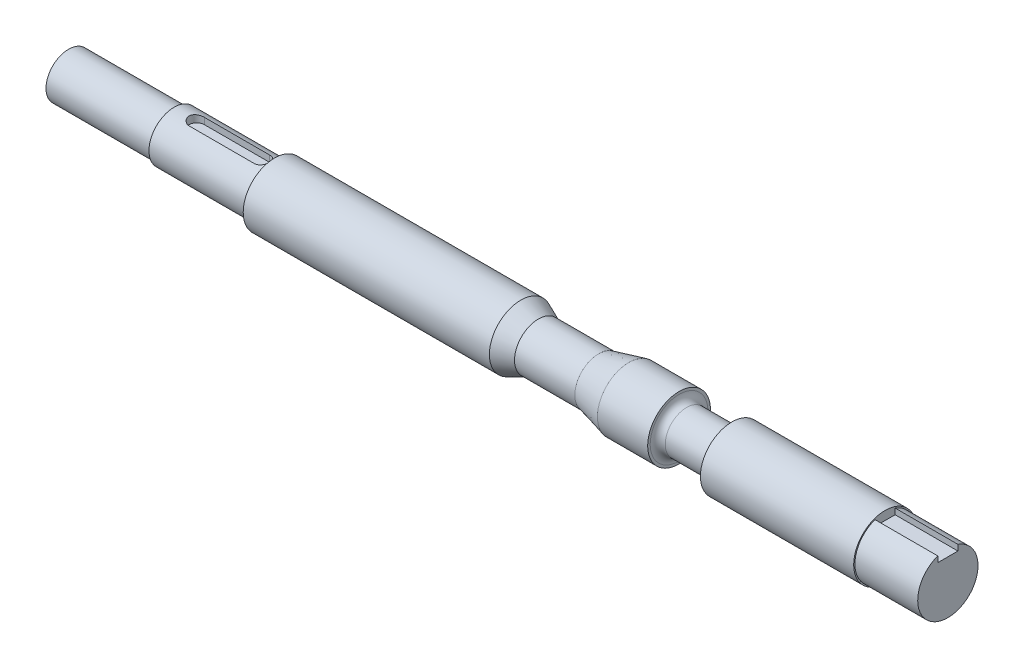
SolidWorks part; units mm, degrees
material "Plain Carbon Steel"
ref_plane "Front Plane" through (0, 0, 0) normal (0, 0, 1) x (1, 0, 0)
ref_plane "Top Plane" through (0, 0, 0) normal (0, 1, 0) x (1, 0, 0)
ref_plane "Right Plane" through (0, 0, 0) normal (1, 0, 0) x (0, 0, -1)
sketch "Shaft Profile Sketch" plane through (0, 0, 0) normal (0, 0, 1) x (1, 0, 0)
  line L0 (0, 0) -> (350, 0)
  line L1 (350, 0) -> (350, 12)
  line L2 (350, 12) -> (325, 12)
  line L3 (325, 12) -> (325, 12.5)
  line L4 (325, 12.5) -> (264, 12.5)
  line L5 (243, 12.5) -> (243, 8.5)
  line L6 (243, 8.5) -> (264, 8.5)
  line L7 (264, 8.5) -> (264, 12.5)
  line L8 (243, 12.5) -> (223, 12.5)
  line L9 (223, 12.5) -> (211, 9.5)
  line L10 (211, 9.5) -> (187, 9.5)
  line L11 (187, 9.5) -> (180, 12.5)
  line L12 (180, 12.5) -> (82, 12.5)
  line L13 (82, 12.5) -> (82, 10)
  line L14 (82, 10) -> (42, 10)
  line L15 (42, 10) -> (42, 9)
  line L16 (42, 9) -> (0, 9)
  line L17 (0, 9) -> (0, 0)
  dimension "D1" = 350
  dimension "D2" = 12
  dimension "D3" = 12.5
  dimension "D4" = 8.5
  dimension "D5" = 9
  dimension "D6" = 10
  dimension "D7" = 9.5
  dimension "D8" = 86
  dimension "D9" = 25
  dimension "D10" = 107
  dimension "D11" = 20
  dimension "D12" = 12
  dimension "D13" = 31
  dimension "D14" = 7
  dimension "D15" = 98
  dimension "D16" = 40
revolve "Shaft Body Revolve" add sketch "Shaft Profile Sketch" angle 360 about L0
fillet "Shoulder Fillet R2" radius 2 1 edges at (264, 0, 8.5)
fillet "Shoulder Fillet R3" radius 3 1 edges at (243, 0, 8.5)
sketch "Keyway A Sketch" plane through (350, 0, 0) normal (1, 0, 0) x (0, 0, -1)
  line L1 (-4, 9) -> (4, 9)
  line L2 (-4, 9) -> (-4, 15)
  line L3 (-4, 15) -> (4, 15)
  line L4 (4, 9) -> (4, 15)
  line L5 (-4, 9) -> (4, 15) construction
  line L6 (-4, 15) -> (4, 9) construction
  circle A0 centre (0, 0) radius 12 construction
  circle A1 centre (0, 0) radius 12 construction
  point P0 (0, 12)
  dimension "D1" = 8
  dimension "D2" = 3
extrude "Keyway A Cut" cut sketch "Keyway A Sketch" against normal up to surface (25 mm away) up to face at (325, 0, 12.5)
sketch "Keyway B Sketch 26x3" plane through (0, 0, 0) normal (0, 1, 0) x (1, 0, 0)
  line L0 (51, 0) -> (77, 0) construction
  line L1 (51, 3) -> (77, 3)
  line L2 (51, -3) -> (77, -3)
  line L3 (42, 10) -> (42, -10) construction
  arc A0 (51, 3) -> (51, -3) centre (51, 0) ccw
  arc A1 (77, -3) -> (77, 3) centre (77, 0) ccw
  point P2 (64, 0)
  dimension "D3" = 3
  dimension "D1" = 26
  dimension "D2" = 9
extrude "Keyway B Cut 26x3" cut sketch "Keyway B Sketch 26x3" against normal blind 3 from offset 10
